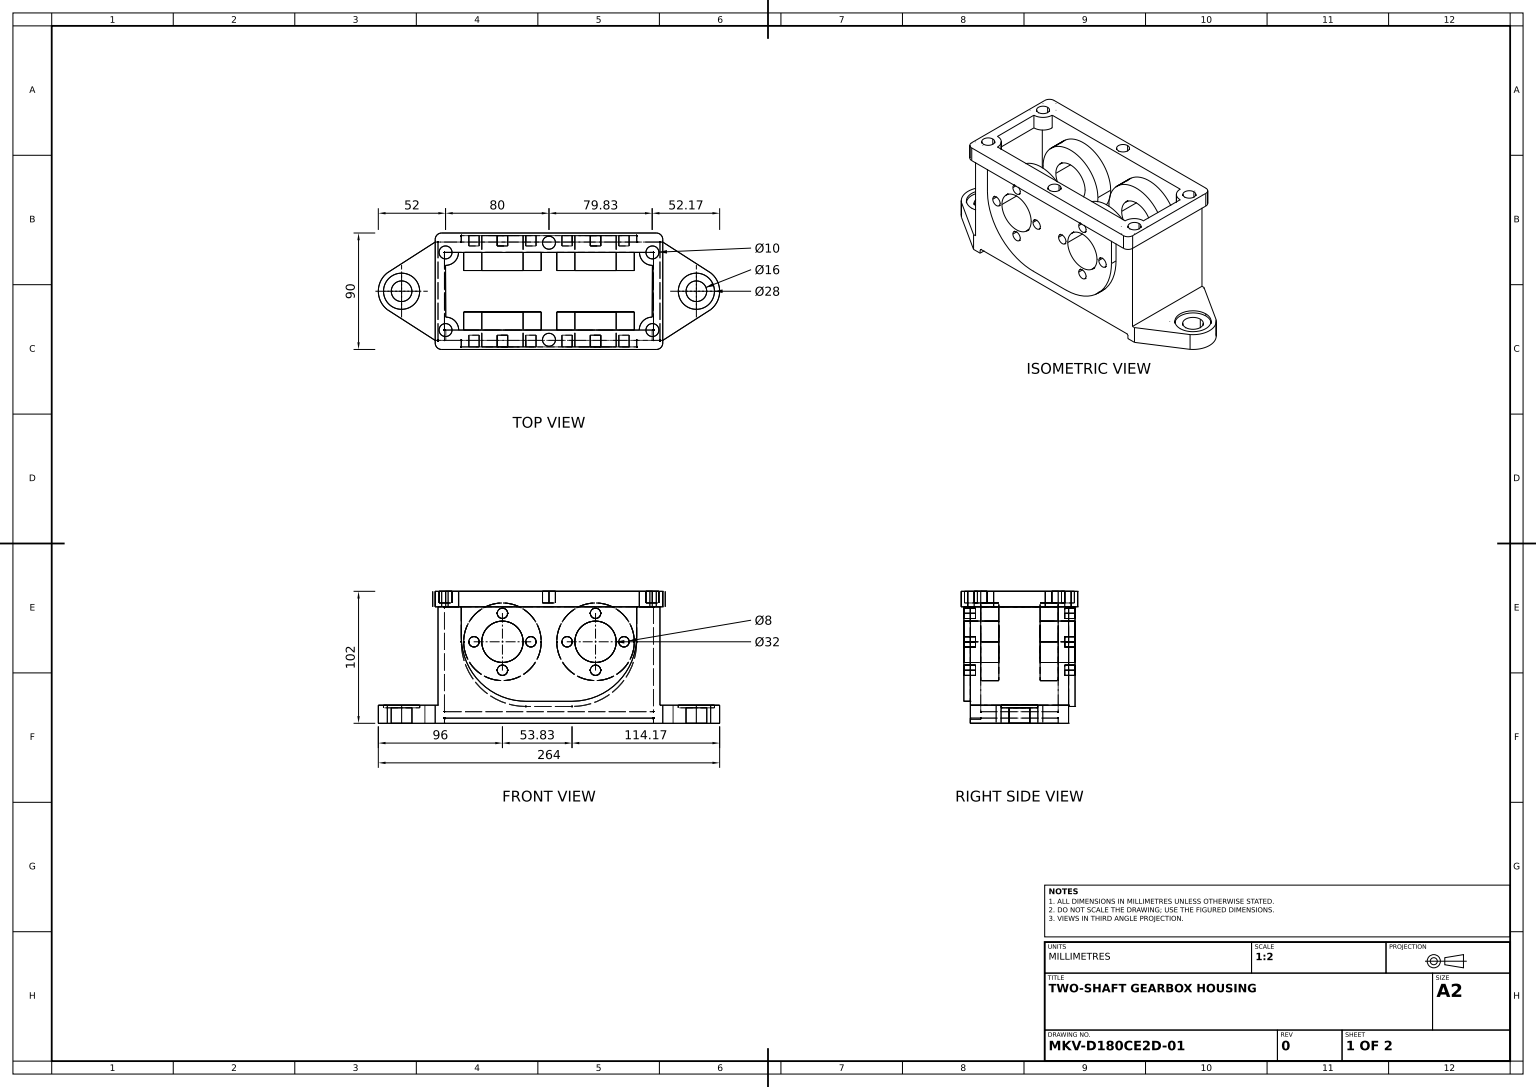
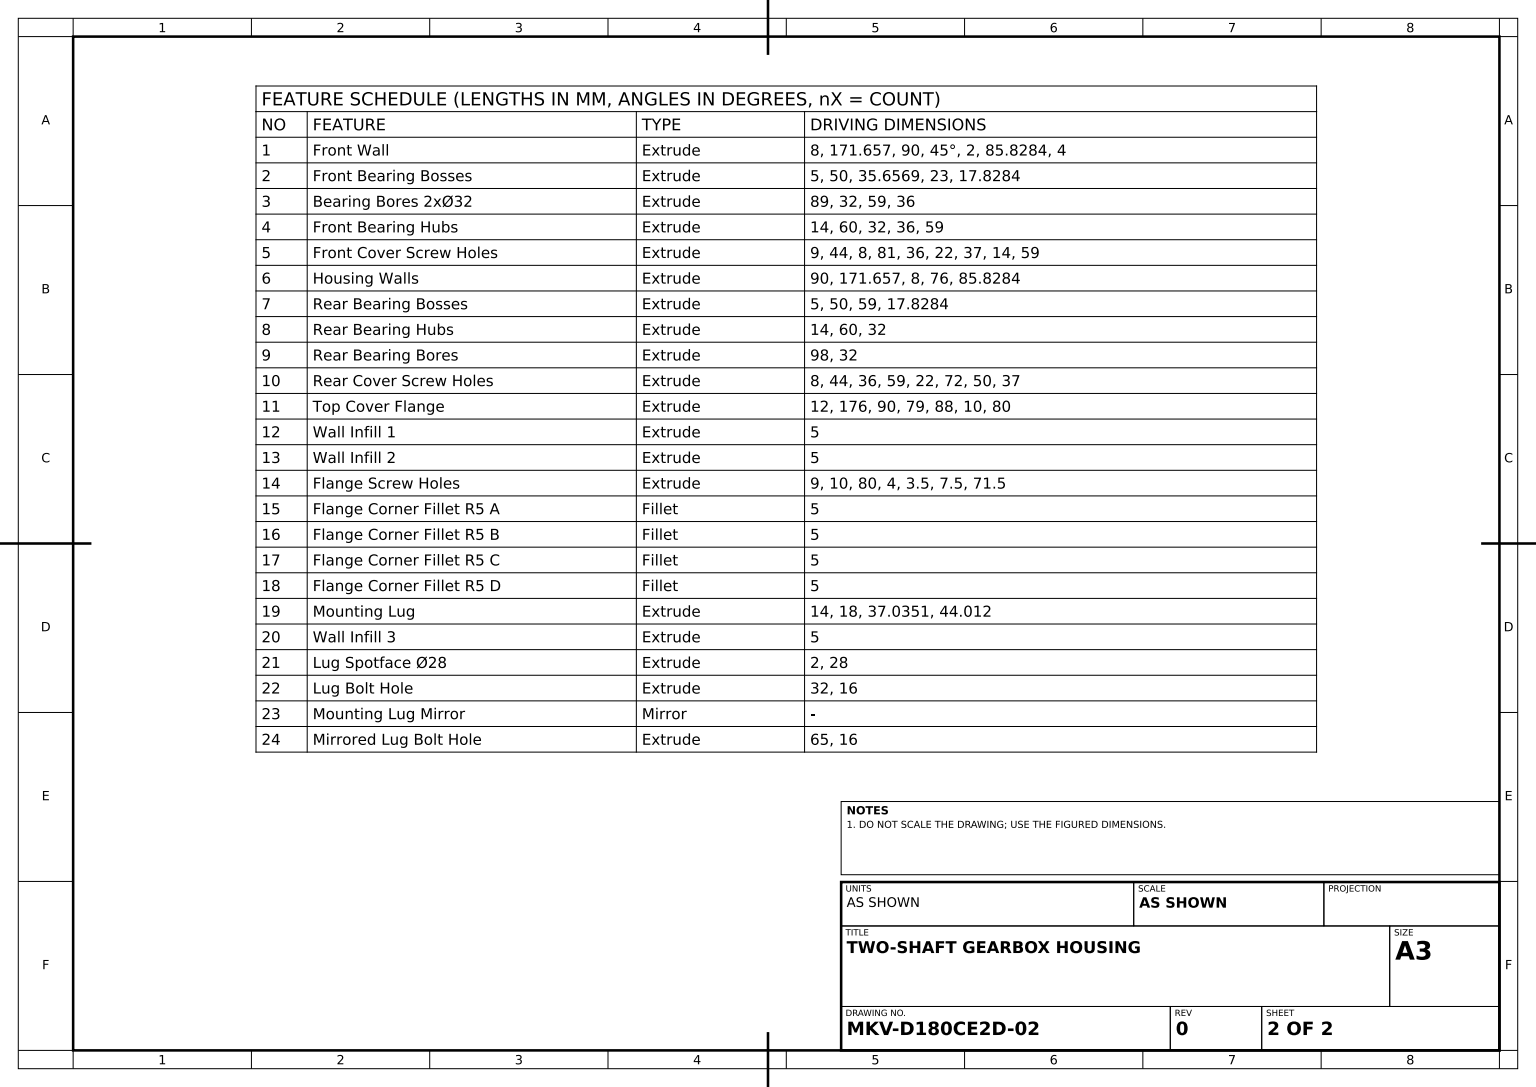
from build123d import *
from build123d.topology import SkipClean

# Parameters (mm, degrees)
FRONT_WALL_DEPTH                = 4
FRONT_BEARING_BOSSES_DEPTH      = 5
BEARING_BORE_SKETCH_R           = 16
BEARING_BORES_2X_32_DEPTH       = 89
FRONT_BEARING_HUB_SKETCH_R      = 30
FRONT_BEARING_HUB_SKETCH_R_2    = 16
FRONT_BEARING_HUBS_DEPTH        = 14
FRONT_COVER_SCREW_HOLE_SKETCH_R = 4
FRONT_COVER_SCREW_HOLES_DEPTH   = 9
HOUSING_WALL_SKETCH_W           = 171.65685425
HOUSING_WALL_SKETCH_H           = 8
HOUSING_WALLS_DEPTH             = 90
REAR_BEARING_BOSSES_DEPTH       = 5
REAR_START                      = 14
REAR_BEARING_HUB_SKETCH_R       = 30
REAR_BEARING_HUB_SKETCH_R_2     = 16
REAR_BEARING_HUBS_DEPTH         = 14
REAR_BEARING_BORE_SKETCH_R      = 16
REAR_BEARING_BORES_DEPTH        = 98
REAR_START_2                    = -8
REAR_COVER_SCREW_HOLE_SKETCH_R  = 4
REAR_COVER_SCREW_HOLES_DEPTH    = 8
TOP_COVER_FLANGE_SKETCH_W       = 176
TOP_COVER_FLANGE_SKETCH_H       = 90
TOP_COVER_FLANGE_DEPTH          = 12
WALL_INFILL_1_SKETCH_W          = 76
WALL_INFILL_1_SKETCH_H          = 102
WALL_INFILL_1_DEPTH             = 5
WALL_INFILL_2_SKETCH_W          = 76
WALL_INFILL_2_SKETCH_H          = 102
WALL_INFILL_2_DEPTH             = 5
FLANGE_SCREW_HOLE_SKETCH_R      = 5
FLANGE_SCREW_HOLES_DEPTH        = 9
FLANGE_CORNER_FILLET_R5_A_R     = 5
FLANGE_CORNER_FILLET_R5_B_R     = 5
FLANGE_CORNER_FILLET_R5_C_R     = 5
FLANGE_CORNER_FILLET_R5_D_R     = 5
MOUNTING_LUG_DEPTH              = 14
WALL_INFILL_3_SKETCH_W          = 161.65685425
WALL_INFILL_3_SKETCH_H          = 68
WALL_INFILL_3_DEPTH             = 5
LUG_SPOTFACE_SKETCH_R           = 14
LUG_SPOTFACE_28_DEPTH           = 2
LUG_BOLT_HOLE_SKETCH_R          = 8
LUG_BOLT_HOLE_DEPTH             = 32
MIRRORED_LUG_BOLT_HOLE_SKETCH_R = 8
MIRRORED_LUG_BOLT_HOLE_DEPTH    = 65


with BuildPart() as part:
    # Front Wall Sketch → Front Wall (new, symmetric)
    with BuildSketch(Plane.XY):
        Polygon((0, 0), (79.828427125, 0), (83.828427125, -4), (85.828427125, -4), (85.828427125, 86), (-85.828427125, 86), (-85.828427125, -4), (-83.828427125, -4), (-79.828427125, 0), align=None)
    extrude(amount=FRONT_WALL_DEPTH, both=True)

    # Front Bearing Boss Sketch → Front Bearing Bosses (add)
    with BuildSketch(Plane.XY.offset(4)):
        with BuildLine():
            Line((-67.828427125, 86), (67.828427125, 86))
            Line((67.828427125, 86), (67.828427125, 63))
            ThreePointArc((67.828427125, 63), (53.183766184, 27.644660941), (17.828427125, 13))
            Line((17.828427125, 13), (-17.828427125, 13))
            ThreePointArc((-17.828427125, 13), (-53.183766184, 27.644660941), (-67.828427125, 63))
            Line((-67.828427125, 63), (-67.828427125, 86))
        make_face()
    extrude(amount=FRONT_BEARING_BOSSES_DEPTH)

    # Bearing Bore Sketch → Bearing Bores 2x_32 (cut)
    with BuildSketch(Plane.XY.offset(9)):
        with Locations((-36, 59)):
            Circle(BEARING_BORE_SKETCH_R)
        with Locations(Location((36, 59, 0), (0, 0, 180))):
            Circle(BEARING_BORE_SKETCH_R)
    extrude(amount=-BEARING_BORES_2X_32_DEPTH, mode=Mode.SUBTRACT)

    # Front Bearing Hub Sketch → Front Bearing Hubs (add)
    # profile 1 of 2: a face of its own
    with SkipClean():  # the faces are left unmerged after this step: merging them gives an invalid solid
        with BuildSketch(Plane(origin=(0, 0, -4), x_dir=(-1, 0, 0), z_dir=(0, 0, -1))):
            with Locations(Location((36, 59, 0), (0, 0, 115.841932763))):
                Circle(FRONT_BEARING_HUB_SKETCH_R)
            with Locations(Location((36, 59, 0), (0, 0, 180))):
                Circle(FRONT_BEARING_HUB_SKETCH_R_2, mode=Mode.SUBTRACT)
        # profile 2 of 2: a face of its own
        with BuildSketch(Plane(origin=(0, 0, -4), x_dir=(-1, 0, 0), z_dir=(0, 0, -1))):
            with Locations(Location((-36, 59, 0), (0, 0, 180))):
                Circle(FRONT_BEARING_HUB_SKETCH_R)
            with Locations(Location((-36, 59, 0), (0, 0, 180))):
                Circle(FRONT_BEARING_HUB_SKETCH_R_2, mode=Mode.SUBTRACT)
        extrude(amount=FRONT_BEARING_HUBS_DEPTH)

    # Front Cover Screw Hole Sketch → Front Cover Screw Holes (cut)
    with SkipClean():  # the faces are left unmerged after this step: merging them gives an invalid solid
        with BuildSketch(Plane.XY.offset(9)):
            with Locations((-36, 81)):
                Circle(FRONT_COVER_SCREW_HOLE_SKETCH_R)
            with Locations((-14, 59)):
                Circle(FRONT_COVER_SCREW_HOLE_SKETCH_R)
            with Locations((-36, 37)):
                Circle(FRONT_COVER_SCREW_HOLE_SKETCH_R)
            with Locations((-58, 59)):
                Circle(FRONT_COVER_SCREW_HOLE_SKETCH_R)
            with Locations(Location((36, 37, 0), (0, 0, 180))):
                Circle(FRONT_COVER_SCREW_HOLE_SKETCH_R)
            with Locations(Location((58, 59, 0), (0, 0, 180))):
                Circle(FRONT_COVER_SCREW_HOLE_SKETCH_R)
            with Locations(Location((36, 81, 0), (0, 0, 180))):
                Circle(FRONT_COVER_SCREW_HOLE_SKETCH_R)
            with Locations(Location((14, 59, 0), (0, 0, 180))):
                Circle(FRONT_COVER_SCREW_HOLE_SKETCH_R)
        extrude(amount=-FRONT_COVER_SCREW_HOLES_DEPTH, mode=Mode.SUBTRACT)



with BuildPart() as body_2:
    # Housing Wall Sketch → Housing Walls (new body)
    with BuildSketch(Plane(origin=(0, 86, 0), x_dir=(1, 0, 0), z_dir=(0, 1, 0))):
        with Locations((0, 68)):
            Rectangle(HOUSING_WALL_SKETCH_W, HOUSING_WALL_SKETCH_H)
    extrude(amount=-HOUSING_WALLS_DEPTH)

    # Rear Bearing Boss Sketch → Rear Bearing Bosses (add)
    with BuildSketch(Plane(origin=(0, 0, -72), x_dir=(-1, 0, 0), z_dir=(0, 0, -1))):
        with BuildLine():
            Line((-67.828427125, 86), (-67.828427125, 59))
            ThreePointArc((-67.828427125, 59), (-53.183766184, 23.644660941), (-17.828427125, 9))
            Line((-17.828427125, 9), (17.828427125, 9))
            ThreePointArc((17.828427125, 9), (53.183766184, 23.644660941), (67.828427125, 59))
            Line((67.828427125, 59), (67.828427125, 86))
            Line((67.828427125, 86), (-67.828427125, 86))
        make_face()
    extrude(amount=REAR_BEARING_BOSSES_DEPTH)

    # Rear Bearing Hub Sketch → Rear Bearing Hubs (add)
    # profile 1 of 2: a face of its own
    with BuildSketch(Plane.XY.offset(-64).offset(REAR_START)):
        with Locations((36, 59)):
            Circle(REAR_BEARING_HUB_SKETCH_R)
        with Locations((36, 59)):
            Circle(REAR_BEARING_HUB_SKETCH_R_2, mode=Mode.SUBTRACT)
    # profile 2 of 2: a face of its own
    with BuildSketch(Plane.XY.offset(-64).offset(REAR_START)):
        with Locations(Location((-36, 59, 0), (0, 0, 64.158067237))):
            Circle(REAR_BEARING_HUB_SKETCH_R)
        with Locations((-36, 59)):
            Circle(REAR_BEARING_HUB_SKETCH_R_2, mode=Mode.SUBTRACT)
    extrude(amount=-REAR_BEARING_HUBS_DEPTH)

    # Rear Bearing Bore Sketch → Rear Bearing Bores (cut)
    with BuildSketch(Plane.XY.offset(-64)):
        with Locations((36, 59)):
            Circle(REAR_BEARING_BORE_SKETCH_R)
        with Locations((-36, 59)):
            Circle(REAR_BEARING_BORE_SKETCH_R)
    extrude(amount=-REAR_BEARING_BORES_DEPTH, mode=Mode.SUBTRACT)

    # Rear Cover Screw Hole Sketch → Rear Cover Screw Holes (cut)
    with BuildSketch(Plane(origin=(0, 0, -77), x_dir=(-1, 0, 0), z_dir=(0, 0, -1)).offset(REAR_START_2)):
        with Locations(Location((36, 81, 0), (0, 0, 180))):
            Circle(REAR_COVER_SCREW_HOLE_SKETCH_R)
        with Locations(Location((58, 59, 0), (0, 0, 180))):
            Circle(REAR_COVER_SCREW_HOLE_SKETCH_R)
        with Locations(Location((36, 37, 0), (0, 0, 180))):
            Circle(REAR_COVER_SCREW_HOLE_SKETCH_R)
        with Locations(Location((14, 59, 0), (0, 0, 180))):
            Circle(REAR_COVER_SCREW_HOLE_SKETCH_R)
        with Locations((-14, 59)):
            Circle(REAR_COVER_SCREW_HOLE_SKETCH_R)
        with Locations((-36, 37)):
            Circle(REAR_COVER_SCREW_HOLE_SKETCH_R)
        with Locations((-58, 59)):
            Circle(REAR_COVER_SCREW_HOLE_SKETCH_R)
        with Locations((-36, 81)):
            Circle(REAR_COVER_SCREW_HOLE_SKETCH_R)
    extrude(amount=REAR_COVER_SCREW_HOLES_DEPTH, mode=Mode.SUBTRACT)


with BuildPart() as part_1:
    with SkipClean():  # the faces are left unmerged after this step: merging them gives an invalid solid
        add(part.part)

        add(body_2.part)  # Top Cover Flange merges body 2
        # Top Cover Flange Sketch → Top Cover Flange (add)
        with BuildSketch(Plane(origin=(0, 86, 0), x_dir=(1, 0, 0), z_dir=(0, 1, 0))):
            with Locations((0, 34)):
                Rectangle(TOP_COVER_FLANGE_SKETCH_W, TOP_COVER_FLANGE_SKETCH_H)
            with BuildLine():
                Line((-69.828427125, 4), (69.828427125, 4))
                ThreePointArc((69.828427125, 4), (72.757359313, 11.071067812), (79.828427125, 14))
                Line((79.828427125, 14), (80, 54))
                ThreePointArc((80, 54), (72.928932188, 56.928932188), (70, 64))
                Line((70, 64), (-70, 64))
                ThreePointArc((-70, 64), (-72.928932188, 56.928932188), (-80, 54))
                Line((-80, 54), (-79.828427125, 14))
                ThreePointArc((-79.828427125, 14), (-72.757359313, 11.071067812), (-69.828427125, 4))
            make_face(mode=Mode.SUBTRACT)
        extrude(amount=TOP_COVER_FLANGE_DEPTH)

    # Wall Infill 1 Sketch → Wall Infill 1 (add)
    with SkipClean():  # the faces are left unmerged after this step: merging them gives an invalid solid
        with BuildSketch(Plane(origin=(85.828427125, 0, 0), x_dir=(0, 0, -1), z_dir=(1, 0, 0))):
            with Locations((34, 47)):
                Rectangle(WALL_INFILL_1_SKETCH_W, WALL_INFILL_1_SKETCH_H)
        extrude(amount=-WALL_INFILL_1_DEPTH)

    # Wall Infill 2 Sketch → Wall Infill 2 (add)
    with SkipClean():  # the faces are left unmerged after this step: merging them gives an invalid solid
        with BuildSketch(Plane.ZY.offset(85.828427125)):
            with Locations((-34, 47)):
                Rectangle(WALL_INFILL_2_SKETCH_W, WALL_INFILL_2_SKETCH_H)
        extrude(amount=-WALL_INFILL_2_DEPTH)

    # Flange Screw Hole Sketch → Flange Screw Holes (cut)
    with SkipClean():  # the faces are left unmerged after this step: merging them gives an invalid solid
        with BuildSketch(Plane(origin=(0, 98, 0), x_dir=(1, 0, 0), z_dir=(0, 1, 0))):
            with Locations(Location((-80, 64, 0), (0, 0, 270))):
                Circle(FLANGE_SCREW_HOLE_SKETCH_R)
            with Locations(Location((0, 71.5, 0), (0, 0, 270))):
                Circle(FLANGE_SCREW_HOLE_SKETCH_R)
            with Locations(Location((80, 64, 0), (0, 0, 270))):
                Circle(FLANGE_SCREW_HOLE_SKETCH_R)
            with Locations(Location((-80, 4, 0), (0, 0, 90))):
                Circle(FLANGE_SCREW_HOLE_SKETCH_R)
            with Locations(Location((0, -3.5, 0), (0, 0, 90))):
                Circle(FLANGE_SCREW_HOLE_SKETCH_R)
            with Locations(Location((80, 4, 0), (0, 0, 90))):
                Circle(FLANGE_SCREW_HOLE_SKETCH_R)
        extrude(amount=-FLANGE_SCREW_HOLES_DEPTH, mode=Mode.SUBTRACT)

    # Flange Corner Fillet R5 A
    flange_corner_fillet_r5_a_edges = [part_1.edges().sort_by_distance(p)[0] for p in [
        (88, 92, 11),
    ]]
    fillet(flange_corner_fillet_r5_a_edges, radius=FLANGE_CORNER_FILLET_R5_A_R)

    # Flange Corner Fillet R5 B
    flange_corner_fillet_r5_b_edges = [part_1.edges().sort_by_distance(p)[0] for p in [
        (88, 92, -79),
    ]]
    fillet(flange_corner_fillet_r5_b_edges, radius=FLANGE_CORNER_FILLET_R5_B_R)

    # Flange Corner Fillet R5 C
    flange_corner_fillet_r5_c_edges = [part_1.edges().sort_by_distance(p)[0] for p in [
        (-88, 92, 11),
    ]]
    fillet(flange_corner_fillet_r5_c_edges, radius=FLANGE_CORNER_FILLET_R5_C_R)

    # Flange Corner Fillet R5 D
    flange_corner_fillet_r5_d_edges = [part_1.edges().sort_by_distance(p)[0] for p in [
        (-88, 92, -79),
    ]]
    fillet(flange_corner_fillet_r5_d_edges, radius=FLANGE_CORNER_FILLET_R5_D_R)

    # Mounting Lug Sketch → Mounting Lug (add)
    with SkipClean():  # the faces are left unmerged after this step: merging them gives an invalid solid
        with BuildSketch(Plane.XZ.offset(4)):
            with BuildLine():
                Line((88, -72), (85.828427125, -72))
                Line((85.828427125, -72), (85.828427125, 4))
                Line((85.828427125, 4), (88, 4))
                Line((88, 4), (125.035091127, -19.779354311))
                ThreePointArc((125.035091127, -19.779354311), (132, -34), (125.035091127, -48.220645689))
                Line((125.035091127, -48.220645689), (88, -72))
            make_face()
        mounting_lug = extrude(amount=-MOUNTING_LUG_DEPTH)

    # Wall Infill 3 Sketch → Wall Infill 3 (add)
    with SkipClean():  # the faces are left unmerged after this step: merging them gives an invalid solid
        with BuildSketch(Plane.XZ):
            with Locations((0, -30)):
                Rectangle(WALL_INFILL_3_SKETCH_W, WALL_INFILL_3_SKETCH_H)
        extrude(amount=-WALL_INFILL_3_DEPTH)

    # Lug Spotface Sketch → Lug Spotface _28 (cut)
    with SkipClean():  # the faces are left unmerged after this step: merging them gives an invalid solid
        with BuildSketch(Plane(origin=(0, 10, 0), x_dir=(1, 0, 0), z_dir=(0, 1, 0))):
            with Locations(Location((114, 34, 0), (0, 0, 270))):
                Circle(LUG_SPOTFACE_SKETCH_R)
        lug_spotface_28 = extrude(amount=-LUG_SPOTFACE_28_DEPTH, mode=Mode.SUBTRACT)

    # Lug Bolt Hole Sketch → Lug Bolt Hole (cut)
    with SkipClean():  # the faces are left unmerged after this step: merging them gives an invalid solid
        with BuildSketch(Plane(origin=(0, 8, 0), x_dir=(1, 0, 0), z_dir=(0, 1, 0))):
            with Locations(Location((114, 34, 0), (0, 0, 270))):
                Circle(LUG_BOLT_HOLE_SKETCH_R)
        extrude(amount=-LUG_BOLT_HOLE_DEPTH, mode=Mode.SUBTRACT)

    # Mounting Lug Mirror: Mounting Lug, Lug Spotface _28 across plane
    with SkipClean():  # the faces are left unmerged after this step: merging them gives an invalid solid
        add(mounting_lug.mirror(Plane(origin=(0, 0, 0), x_dir=(0, 0, 1), z_dir=(1, 0, 0))))
        add(lug_spotface_28.mirror(Plane(origin=(0, 0, 0), x_dir=(0, 0, 1), z_dir=(1, 0, 0))), mode=Mode.SUBTRACT)

    # Mirrored Lug Bolt Hole Sketch → Mirrored Lug Bolt Hole (cut)
    with SkipClean():  # the faces are left unmerged after this step: merging them gives an invalid solid
        with BuildSketch(Plane(origin=(0, 8, 0), x_dir=(1, 0, 0), z_dir=(0, 1, 0))):
            with Locations(Location((-114, 34, 0), (0, 0, 270))):
                Circle(MIRRORED_LUG_BOLT_HOLE_SKETCH_R)
        extrude(amount=-MIRRORED_LUG_BOLT_HOLE_DEPTH, mode=Mode.SUBTRACT)


solid = part_1.part
